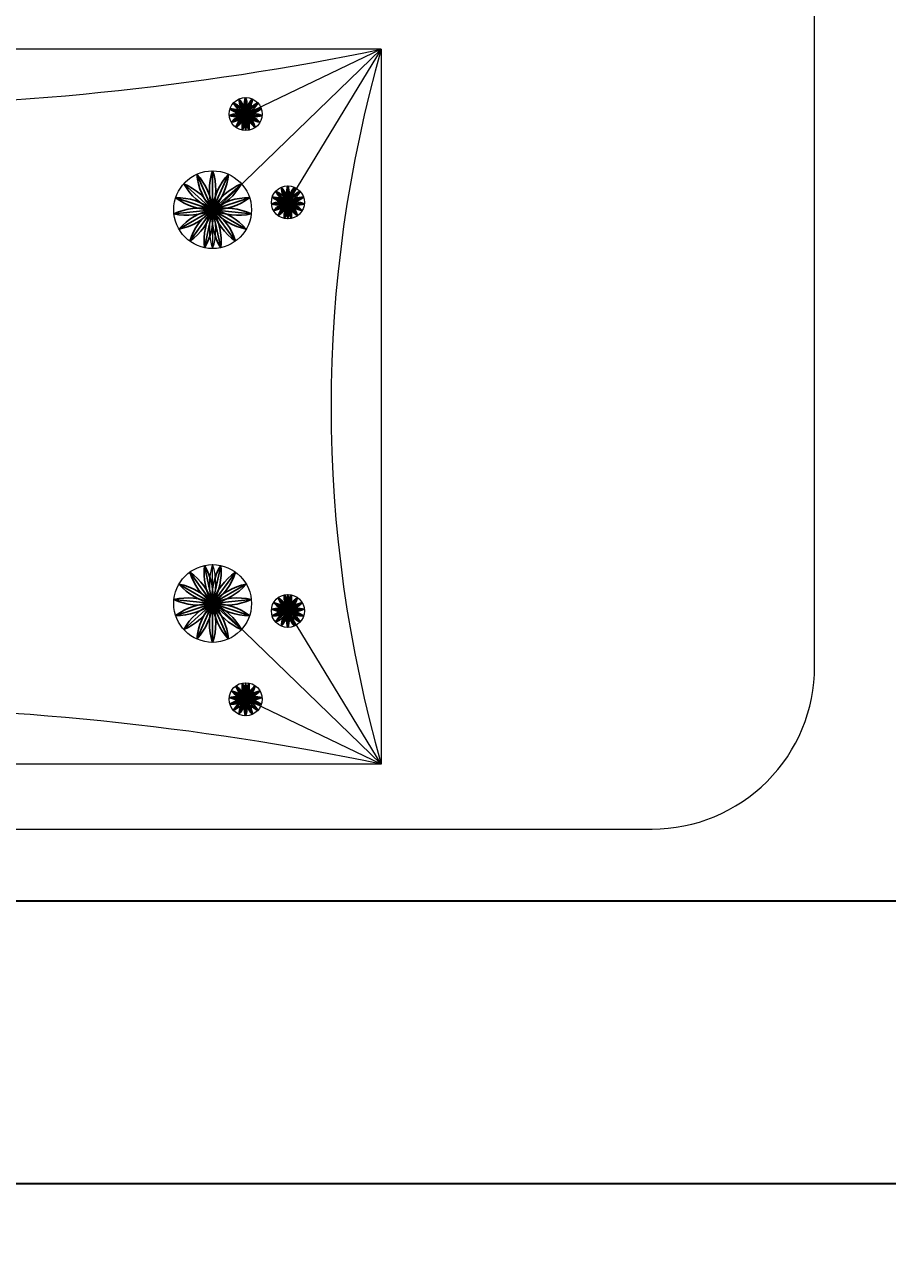
# Model space of a CAD drawing. Units: inches. Extents: x -61 to 1599, y -1316 to 257.
# Tile 37 of 204: x 152 to 171, y -790 to -763. Entities that reach past the tile are written whole.
import ezdxf

# ---------------------------------------------------------------- set-up
doc = ezdxf.new("R2010")
doc.units = ezdxf.units.IN
doc.header["$MEASUREMENT"] = 0
for name, color, linetype, lineweight in [('A-ANNO-DIMS', 2, 'Continuous', 18), ('FURNITURE', 83, 'Continuous', 18), ('WALLS', 4, 'Continuous', 35)]:
    doc.layers.add(name, color=color, linetype=linetype, lineweight=lineweight)
doc.layers.add('LT', color=8, linetype='Continuous')
doc.styles.get("Standard").update_dxf_attribs({"font": 'arial.ttf'})
doc.dimstyles.get("Standard").update_dxf_attribs({"dimtxt": 0.18, "dimasz": 0.18, "dimexe": 0.18, "dimexo": 0.0625, "dimgap": 0.09, "dimtad": 0, "dimtih": 1, "dimtoh": 1, "dimdec": 0, "dimzin": 0, "dimdsep": 46, "dimlunit": 3, "dimtxsty": 'Standard', "dimcen": 0.09, "dimadec": 0, "dimazin": 0, "dimtfac": 1, "dimtdec": 0, "dimtofl": 0, "dimtmove": 0, "dimatfit": 3, "dimfxl": 1, "dimtolj": 1, "dimtzin": 0, "dimarcsym": 0})

# ---------------------------------------------------------------- blocks, each defined once
blk = doc.blocks.new('*U42')
at = {"layer": 'LT'}
blk.add_line((0, 0.412), (0, -0.412), dxfattribs=at)
for centre, start, end in [((1.198, 0), 160.9983, 199.0017), ((-1.198, 0), 340.9983, 19.0017)]:
    blk.add_arc(centre, 1.267, start, end, dxfattribs=at)
blk = doc.blocks.new('*U43')
at = {"layer": 'LT', "transparency": 16777216}
for p, rotation in [((-156.639, -43.959), 48.00000000000001), ((-156.501, -43.858), 24), ((-156.165, -43.858), 336.0000000000001), ((-156.027, -43.959), 312), ((-156.743, -44.278), 96), ((-156.725, -44.108), 72), ((-156.69, -44.441), 120), ((-155.976, -44.441), 240), ((-155.941, -44.108), 288.0000000000001), ((-155.923, -44.278), 264), ((-156.575, -44.569), 144), ((-156.419, -44.639), 168), ((-156.247, -44.639), 192), ((-156.091, -44.569), 216)]:
    blk.add_blockref('*U42', p, dxfattribs=dict(at, rotation=rotation))
blk.add_blockref('*U42', (-156.333, -43.823), dxfattribs=at)
blk = doc.blocks.new('*U31')
at = {"layer": 'LT'}
blk.add_line((0, 0.412), (0, -0.412), dxfattribs=at)
for centre, start, end in [((1.198, 0), 160.9983, 199.0017), ((-1.198, 0), 340.9983, 19.0017)]:
    blk.add_arc(centre, 1.267, start, end, dxfattribs=at)
blk = doc.blocks.new('*U32')
at = {"layer": 'LT', "transparency": 16777216}
for p, rotation in [((-156.639, -43.959), 48.00000000000001), ((-156.501, -43.858), 24), ((-156.165, -43.858), 336.0000000000001), ((-156.027, -43.959), 312), ((-156.743, -44.278), 96), ((-156.725, -44.108), 72), ((-156.69, -44.441), 120), ((-155.976, -44.441), 240), ((-155.941, -44.108), 288.0000000000001), ((-155.923, -44.278), 264), ((-156.575, -44.569), 144), ((-156.419, -44.639), 168), ((-156.247, -44.639), 192), ((-156.091, -44.569), 216)]:
    blk.add_blockref('*U31', p, dxfattribs=dict(at, rotation=rotation))
blk.add_blockref('*U31', (-156.333, -43.823), dxfattribs=at)
blk = doc.blocks.new('*U48')
at = {"layer": 'LT'}
blk.add_line((0, 0.175), (0, -0.175), dxfattribs=at)
for centre, start, end in [((0.509, 0), 160.9983, 199.0017), ((-0.509, 0), 340.9983, 19.0017)]:
    blk.add_arc(centre, 0.539, start, end, dxfattribs=at)
blk = doc.blocks.new('*U49')
at = {"layer": 'LT', "transparency": 16777216}
for p, rotation in [((-66.605, -18.692), 48.00000000000001), ((-66.546, -18.649), 24), ((-66.404, -18.649), 336.0000000000001), ((-66.345, -18.692), 312), ((-66.649, -18.828), 96), ((-66.642, -18.755), 72), ((-66.627, -18.897), 120), ((-66.578, -18.951), 144), ((-66.512, -18.981), 168.0000000000001), ((-66.439, -18.981), 192), ((-66.372, -18.951), 216), ((-66.323, -18.897), 240), ((-66.308, -18.755), 288.0000000000001), ((-66.301, -18.828), 264)]:
    blk.add_blockref('*U48', p, dxfattribs=dict(at, rotation=rotation))
blk.add_blockref('*U48', (-66.475, -18.634), dxfattribs=at)
blk = doc.blocks.new('*U24')
at = {"layer": 'LT'}
blk.add_line((0, 0.175), (0, -0.175), dxfattribs=at)
for centre, start, end in [((0.509, 0), 160.9983, 199.0017), ((-0.509, 0), 340.9983, 19.0017)]:
    blk.add_arc(centre, 0.539, start, end, dxfattribs=at)
blk = doc.blocks.new('*U25')
at = {"layer": 'LT', "transparency": 16777216}
for p, rotation in [((-66.605, -18.692), 48.00000000000001), ((-66.546, -18.649), 24), ((-66.404, -18.649), 336.0000000000001), ((-66.345, -18.692), 312), ((-66.649, -18.828), 96), ((-66.642, -18.755), 72), ((-66.627, -18.897), 120), ((-66.578, -18.951), 144), ((-66.512, -18.981), 168.0000000000001), ((-66.439, -18.981), 192), ((-66.372, -18.951), 216), ((-66.323, -18.897), 240), ((-66.308, -18.755), 288.0000000000001), ((-66.301, -18.828), 264)]:
    blk.add_blockref('*U24', p, dxfattribs=dict(at, rotation=rotation))
blk.add_blockref('*U24', (-66.475, -18.634), dxfattribs=at)
blk = doc.blocks.new('*U50')
at = {"layer": 'LT'}
blk.add_line((0, 0.175), (0, -0.175), dxfattribs=at)
for centre, start, end in [((0.509, 0), 160.9983, 199.0017), ((-0.509, 0), 340.9983, 19.0017)]:
    blk.add_arc(centre, 0.539, start, end, dxfattribs=at)
blk = doc.blocks.new('*U51')
at = {"layer": 'LT', "transparency": 16777216}
for p, rotation in [((-66.605, -18.692), 48.00000000000001), ((-66.546, -18.649), 24), ((-66.404, -18.649), 336.0000000000001), ((-66.345, -18.692), 312), ((-66.649, -18.828), 96), ((-66.642, -18.755), 72), ((-66.627, -18.897), 120), ((-66.578, -18.951), 144), ((-66.512, -18.981), 168.0000000000001), ((-66.439, -18.981), 192), ((-66.372, -18.951), 216), ((-66.323, -18.897), 240), ((-66.308, -18.755), 288.0000000000001), ((-66.301, -18.828), 264)]:
    blk.add_blockref('*U50', p, dxfattribs=dict(at, rotation=rotation))
blk.add_blockref('*U50', (-66.475, -18.634), dxfattribs=at)
blk = doc.blocks.new('*U26')
at = {"layer": 'LT'}
blk.add_line((0, 0.175), (0, -0.175), dxfattribs=at)
for centre, start, end in [((0.509, 0), 160.9983, 199.0017), ((-0.509, 0), 340.9983, 19.0017)]:
    blk.add_arc(centre, 0.539, start, end, dxfattribs=at)
blk = doc.blocks.new('*U27')
at = {"layer": 'LT', "transparency": 16777216}
for p, rotation in [((-66.605, -18.692), 48.00000000000001), ((-66.546, -18.649), 24), ((-66.404, -18.649), 336.0000000000001), ((-66.345, -18.692), 312), ((-66.649, -18.828), 96), ((-66.642, -18.755), 72), ((-66.627, -18.897), 120), ((-66.578, -18.951), 144), ((-66.512, -18.981), 168.0000000000001), ((-66.439, -18.981), 192), ((-66.372, -18.951), 216), ((-66.323, -18.897), 240), ((-66.308, -18.755), 288.0000000000001), ((-66.301, -18.828), 264)]:
    blk.add_blockref('*U26', p, dxfattribs=dict(at, rotation=rotation))
blk.add_blockref('*U26', (-66.475, -18.634), dxfattribs=at)
blk = doc.blocks.new('BED-DOUBLE')
for p, q in [((61.064, 16.557), (37.147, 16.557)), ((61.064, 16.557), (57.496, 13.107)), ((61.064, 16.557), (58.185, 15.18)), ((61.064, 16.557), (59.081, 13.305)), ((58.185, 15.18), (58.185, 14.829)), ((57.483, 13.149), (57.483, 12.324)), ((59.081, 13.305), (59.081, 12.955)), ((57.483, 4.788), (57.483, 5.613)), ((61.064, 1.379), (57.496, 4.83)), ((59.081, 4.631), (59.081, 4.982)), ((61.064, 1.379), (59.081, 4.631)), ((58.185, 2.756), (58.185, 3.107)), ((61.064, 1.379), (58.185, 2.756)), ((61.064, 1.379), (61.064, 1.379))]:
    blk.add_line(p, q)
for points in [[(1.272, 88.537), (1.272, 3.449, 0.414214), (4.722, 0), (66.813, 0, 0.414214), (70.263, 3.449), (70.263, 88.537, 0.414214), (66.813, 91.987), (4.722, 91.987, 0.414214)], [(57.483, 12.324, 0.167358), (57.483, 13.149, 0.167358)], [(59.081, 12.955, 0.167358), (59.081, 13.305, 0.167358)], [(57.483, 4.788, 0.167358), (57.483, 5.613, 0.167358)], [(59.081, 4.631, 0.167358), (59.081, 4.982, 0.167358)], [(58.185, 2.756, 0.167358), (58.185, 3.107, 0.167358)]]:
    blk.add_lwpolyline(points, format="xyb", close=True)
blk.add_lwpolyline([(61.064, 16.557), (61.064, 1.379), (37.147, 1.379)])
for centre, radius in [((58.185, 15.18), 0.351), ((57.483, 13.149), 0.825), ((59.081, 13.305), 0.351), ((57.483, 4.788), 0.825), ((59.081, 4.631), 0.351), ((58.185, 2.756), 0.351)]:
    blk.add_circle(centre, radius)
for centre, radius, start, end in [((49.106, 74.54), 59.203, 258.34678, 281.65322), ((87.538, 8.968), 27.54, 164.0046, 195.9954), ((58.694, 15.005), 0.539, 160.9983, 199.0017), ((57.675, 15.005), 0.539, 340.9983, 19.0017), ((49.106, -56.603), 59.203, 78.34678, 101.65322)]:
    blk.add_arc(centre, radius, start, end)
at = {"extrusion": (0, 0, -1), "zscale": -1}
for name, p in [('*U25', (8.291, 33.99)), ('*U32', (98.85, 57.384)), ('*U27', (7.394, 32.115))]:
    blk.add_blockref(name, p, dxfattribs=at)
at = {"rotation": 180}
for name, p in [('*U43', (-98.85, -39.447)), ('*U51', (-7.394, -14.178)), ('*U49', (-8.291, -16.053))]:
    blk.add_blockref(name, p, dxfattribs=at)
blk = doc.blocks.new('*D687')
at = {"layer": 'A-ANNO-DIMS', "color": 0, "lineweight": -2, "transparency": 16777216}
for p, q in [((289.418, 181.677), (-61.077, 181.677)), ((-60.897, 181.497), (-60.897, -528.952)), ((-60.897, -1239.765), (-60.897, -529.316)), ((319.64, -1239.945), (-61.077, -1239.945))]:
    blk.add_line(p, q, dxfattribs=at)
at = {"layer": 'A-ANNO-DIMS', "color": 0, "transparency": 16777216}
for points in [[(-60.927, 181.497), (-60.867, 181.497), (-60.897, 181.677)], [(-60.927, -1239.765), (-60.867, -1239.765), (-60.897, -1239.945)]]:
    blk.add_solid(points, dxfattribs=at)
at = {"layer": 'DEFPOINTS', "color": 0, "transparency": 16777216}
for p in [(289.481, 181.677), (-60.897, -1239.945), (319.703, -1239.945)]:
    blk.add_point(p, dxfattribs=at)
at = {"layer": 'A-ANNO-DIMS', "color": 0, "transparency": 16777216, "insert": (-60.897, -529.134), "char_height": 0.18, "attachment_point": 5}
blk.add_mtext('\\A1;1421.6', dxfattribs=at)

msp = doc.modelspace()

# ---------------------------------------------------------------- linework, layer by layer
at = {"layer": 'WALLS'}
for p, q in [((14.7028, -781.9446), (237.7028, -781.9446)), ((14.7028, -787.9446), (237.7028, -787.9446))]:
    msp.add_line(p, q, dxfattribs=at)

# ---------------------------------------------------------------- block references
at = {"layer": 'FURNITURE'}
msp.add_blockref('BED-DOUBLE', (98.977, -780.4187), dxfattribs=at)

# ---------------------------------------------------------------- dimensions: what is measured, and where the dimension line sits
at = {"layer": 'A-ANNO-DIMS'}
dim = msp.add_linear_dim(base=(-60.8972, -1239.9446), p1=(289.4807, 181.6771), p2=(319.7028, -1239.9446), angle=90, dimstyle='Standard', override={"dimdec": 1, "dimlfac": 1, "dimrnd": 0, "dimzin": 0, "dimdsep": 46, "dimlunit": 2}, dxfattribs=at)
dim.commit()
dim.dimension.update_dxf_attribs({"geometry": '*D687', "text_midpoint": (-60.8972, -529.1337)})

doc.saveas('drawing.dxf')
